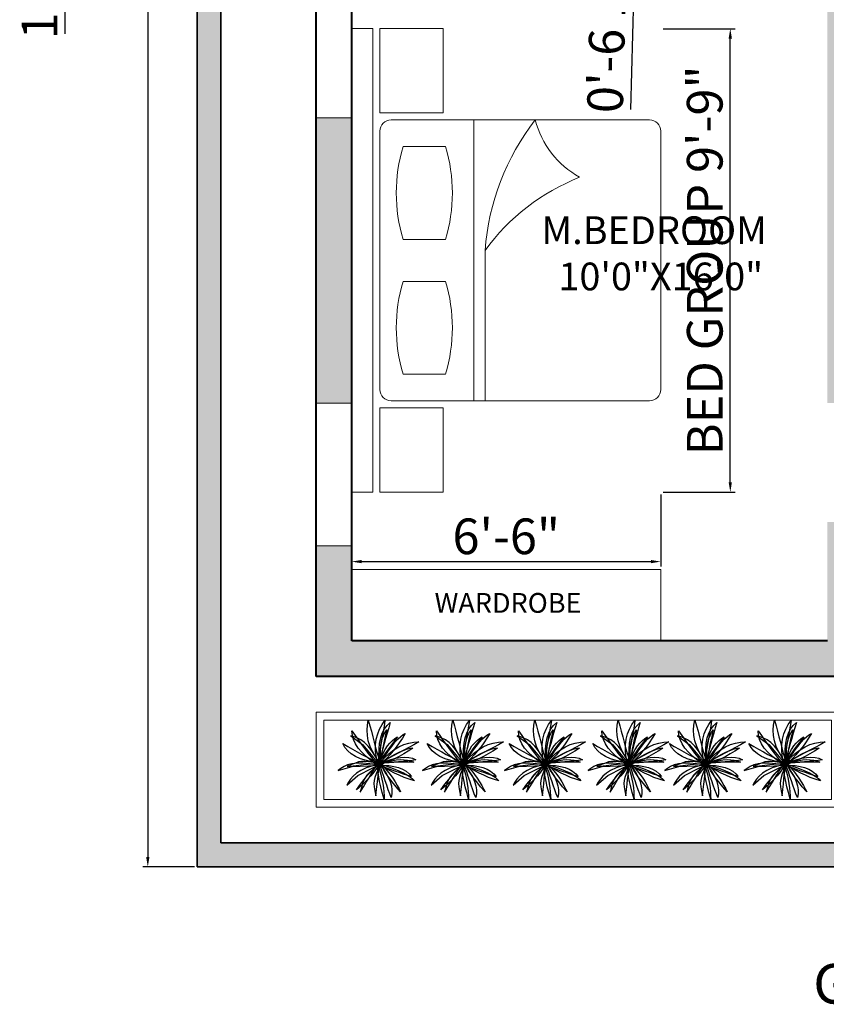
# Model space of a CAD drawing. Units: inches. Extents: x 2337 to 3570, y 1258 to 1938.
# Tile 1 of 30: x 2381 to 2585, y 1258 to 1507. Entities that reach past the tile are written whole.
import ezdxf

# ---------------------------------------------------------------- set-up
doc = ezdxf.new("R2010")
doc.units = ezdxf.units.IN
for name, color, linetype, lineweight in [('A-ANNO-DIMS', 2, 'Continuous', 18), ('A-ANNO-TEXT', 7, 'Continuous', 18), ('A-ANNO-TITL', 7, 'Continuous', 30), ('A-AREA-IDEN', 7, 'Continuous', 18), ('A-FLOR-CASE', 34, 'Continuous', 18), ('A-GLAZ', 4, 'Continuous', 18), ('A-WALL', 7, 'Continuous', 40), ('C-PROP', 7, 'Continuous', 35), ('CAY', 94, 'Continuous', 13), ('furn', 8, 'Continuous', 18), ('L-PLNT-BEDS', 94, 'Continuous', 20)]:
    doc.layers.add(name, color=color, linetype=linetype, lineweight=lineweight)
doc.layers.add('A-WALL-PATT', color=18, linetype='Continuous', lineweight=13, true_color=0x000000)
doc.layers.add('C-PROP-PATT', color=251, linetype='Continuous', lineweight=13, true_color=0x636466)
doc.layers.add('DIENHOA', color=3, linetype='Continuous')
doc.styles.get("Standard").update_dxf_attribs({"font": 'arial.ttf'})
doc.dimstyles.new('ISO-25', dxfattribs={"dimtxt": 9, "dimasz": 2.5, "dimexe": 1.25, "dimexo": 0.625, "dimtad": 1, "dimdec": 1, "dimlunit": 3, "dimtxsty": 'Standard', "dimcen": 2.5, "dimadec": 0, "dimazin": 0, "dimtfac": 1, "dimtdec": 1, "dimtmove": 0, "dimatfit": 3, "dimfxl": 1, "dimarcsym": 0})

# ---------------------------------------------------------------- blocks, each defined once
blk = doc.blocks.new('*D7')
at = {"layer": 'A-ANNO-DIMS', "color": 0, "lineweight": -2, "transparency": 16777216}
for p, q in [((2425.21, 1893.12), (2412.15, 1893.12)), ((2413.4, 1890.62), (2413.4, 1295.62)), ((2425.21, 1293.12), (2412.15, 1293.12))]:
    blk.add_line(p, q, dxfattribs=at)
at = {"layer": 'A-ANNO-DIMS', "color": 0, "transparency": 16777216}
for points in [[(2412.98, 1890.62), (2413.81, 1890.62), (2413.4, 1893.12)], [(2412.98, 1295.62), (2413.81, 1295.62), (2413.4, 1293.12)]]:
    blk.add_solid(points, dxfattribs=at)
at = {"layer": 'Defpoints', "color": 0, "transparency": 16777216}
for p in [(2425.84, 1893.12), (2413.4, 1293.12), (2425.84, 1293.12)]:
    blk.add_point(p, dxfattribs=at)
at = {"layer": 'A-ANNO-DIMS', "color": 0, "transparency": 16777216, "insert": (2408.18, 1593.12), "char_height": 9, "attachment_point": 5, "rotation": 90}
blk.add_mtext("50'", dxfattribs=at)
blk = doc.blocks.new('MAT-P16')
for p, q in [((0, -1.65), (0, 1.65)), ((0, 1.65), (0.15, 1.65)), ((0.15, 1.65), (0.15, -1.65)), ((0.65, 1.65), (0.2, 1.65)), ((0.2, 1.65), (0.2, 1.05)), ((0.65, 1.05), (0.65, 1.65)), ((0.65, 1.05), (0.2, 1.05)), ((2.12, 1), (0.28, 1)), ((0.8695, -1), (0.8695, 1)), ((0.2, 0.92), (0.2, -0.92)), ((2.2, -0.92), (2.2, 0.92)), ((0.6667, 0.8098), (0.3667, 0.8098)), ((0.3667, 0.1498), (0.6667, 0.1498)), ((0.9496, -1), (0.9496, 0.0713)), ((0.3667, -0.1498), (0.6667, -0.1498)), ((0.6667, -0.8098), (0.3667, -0.8098)), ((0.65, -1.05), (0.2, -1.05)), ((0.2, -1.65), (0.2, -1.05)), ((0.28, -1), (2.12, -1)), ((0.65, -1.05), (0.65, -1.65)), ((0.15, -1.65), (0, -1.65)), ((0.65, -1.65), (0.2, -1.65))]:
    blk.add_line(p, q)
for centre, radius, start, end in [((0.28, 0.92), 0.08, 90, 180), ((2.6605, -0.0533), 1.7154, 142.12135, 175.83412), ((1.9461, 1.1681), 0.6614, 194.72006, 240.68633), ((2.12, 0.92), 0.08, 0, 90), ((1.4307, 0.4798), 1.114, 162.7687, 197.2313), ((-0.3973, 0.4798), 1.114, 342.7687, 17.2313), ((2.172, -0.8149), 1.5099, 111.34847, 144.05792), ((1.4307, -0.4798), 1.114, 162.7687, 197.2313), ((-0.3973, -0.4798), 1.114, 342.7687, 17.2313), ((0.28, -0.92), 0.08, 180, 270), ((2.12, -0.92), 0.08, 270, 0)]:
    blk.add_arc(centre, radius, start, end)
blk = doc.blocks.new('Cay03_mb')
at = {"layer": 'DIENHOA'}
for p, q in [((119, 555), (166, 599)), ((166, 599), (142, 519)), ((25, 374), (49, 444)), ((49, 444), (79, 504)), ((79, 504), (119, 555)), ((119, 442), (97, 366)), ((142, 519), (119, 442)), ((-365, 390), (-414, 403)), ((-414, 403), (-240, 278)), ((-315, 371), (-365, 390)), ((-264, 343), (-315, 371)), ((-211, 305), (-264, 343)), ((-158, 252), (-211, 305)), ((2, 206), (10, 295)), ((10, 295), (25, 374)), ((76, 291), (56, 216)), ((97, 366), (76, 291)), ((363, 275), (437, 297)), ((437, 297), (511, 310)), ((511, 310), (586, 314)), ((586, 314), (512, 271)), ((-240, 278), (-88, 95)), ((-104, 184), (-158, 252)), ((-50, 98), (-104, 184)), ((0, 105), (2, 206)), ((56, 216), (37, 142)), ((147, 144), (219, 200)), ((290, 155), (217, 117)), ((219, 200), (291, 243)), ((364, 193), (290, 155)), ((291, 243), (363, 275)), ((438, 231), (364, 193)), ((512, 271), (438, 231)), ((-345, 5), (-400, -17)), ((-299, 20), (-345, 5)), ((-255, 27), (-299, 20)), ((-208, 28), (-255, 27)), ((-153, 22), (-208, 28)), ((-83, 10), (-153, 22)), ((-88, 95), (5, -8)), ((5, -8), (-83, 10)), ((5, -8), (-50, 98)), ((5, -8), (0, 105)), ((5, -8), (76, 75)), ((20, 68), (5, -8)), ((75, 36), (5, -8)), ((5, -8), (100, 18)), ((46, 1), (5, -8)), ((37, 142), (20, 68)), ((97, 7), (46, 1)), ((145, 77), (75, 36)), ((76, 75), (147, 144)), ((155, 12), (97, 7)), ((100, 18), (182, 37)), ((217, 117), (145, 77)), ((220, 15), (155, 12)), ((182, 37), (253, 49)), ((289, 17), (220, 15)), ((253, 49), (315, 54)), ((362, 19), (289, 17)), ((315, 54), (369, 53)), ((436, 19), (362, 19)), ((369, 53), (419, 47)), ((419, 47), (465, 35)), ((510, 19), (436, 19)), ((465, 35), (510, 19)), ((-400, -17), (-468, -48)), ((-468, -48), (-376, -38)), ((-376, -38), (-295, -28)), ((-295, -28), (-226, -19)), ((-226, -19), (-166, -11)), ((-166, -11), (-114, -6)), ((-166, -174), (-120, -122)), ((-120, -122), (-80, -80)), ((-75, -127), (-118, -181)), ((-114, -6), (-69, -3)), ((-80, -80), (-45, -46)), ((-33, -69), (-75, -127)), ((-69, -3), (-30, -3)), ((-45, -46), (-17, -22)), ((5, -8), (-33, -69)), ((-30, -3), (5, -8)), ((-17, -22), (5, -8)), ((5, -8), (57, -73)), ((26, -64), (5, -8)), ((5, -8), (113, -40)), ((53, -42), (5, -8)), ((47, -126), (26, -64)), ((69, -191), (47, -126)), ((107, -76), (53, -42)), ((57, -73), (100, -139)), ((100, -139), (136, -204)), ((166, -110), (107, -76)), ((113, -40), (207, -74)), ((229, -143), (166, -110)), ((207, -74), (290, -108)), ((296, -175), (229, -143)), ((290, -108), (359, -141)), ((359, -141), (417, -174)), ((-271, -307), (-216, -236)), ((-206, -276), (-250, -318)), ((-216, -236), (-166, -174)), ((-162, -231), (-206, -276)), ((-118, -181), (-162, -231)), ((91, -257), (69, -191)), ((113, -322), (91, -257)), ((136, -204), (163, -268)), ((163, -268), (181, -330)), ((367, -205), (296, -175)), ((442, -233), (367, -205)), ((417, -174), (463, -204)), ((519, -258), (442, -233)), ((463, -204), (496, -232)), ((496, -232), (519, -258)), ((-330, -387), (-271, -307)), ((-291, -355), (-330, -387)), ((-250, -318), (-291, -355)), ((135, -386), (113, -322)), ((158, -445), (135, -386)), ((181, -330), (190, -390)), ((190, -390), (190, -446)), ((180, -499), (158, -445)), ((190, -446), (180, -499))]:
    blk.add_line(p, q, dxfattribs=at)
for points in [[(24, -5), (-41, 82), (-92, 167), (-130, 249), (-156, 330), (-170, 408), (-175, 484), (-170, 559), (-157, 633)], [(-157, 633), (-132, 551), (-111, 470), (-90, 389), (-70, 309), (-49, 229), (-27, 150), (-3, 72), (24, -5)], [(-16, -27), (-38, 80), (-49, 178), (-49, 269), (-39, 353), (-19, 430), (9, 501), (45, 567), (88, 629)], [(88, 629), (75, 544), (61, 461), (46, 379), (31, 298), (16, 217), (3, 136), (-8, 55), (-16, -27)], [(-396, 474), (-348, 406), (-301, 339), (-254, 275), (-208, 212), (-162, 151), (-115, 91), (-66, 32), (-16, -27)], [(-16, -27), (-108, 39), (-187, 102), (-252, 163), (-305, 224), (-345, 285), (-374, 347), (-390, 409), (-396, 474)], [(24, -5), (20, 93), (20, 177), (25, 249), (34, 310), (47, 363), (65, 409), (87, 452), (113, 492)], [(113, 492), (96, 420), (79, 347), (64, 276), (50, 208), (38, 145), (30, 87), (25, 36), (24, -5)], [(384, 437), (342, 368), (298, 302), (253, 239), (206, 181), (159, 127), (113, 78), (68, 34), (24, -5)], [(24, -5), (80, 92), (134, 176), (186, 248), (234, 309), (279, 357), (319, 395), (355, 421), (384, 437)], [(-530, 290), (-458, 248), (-388, 208), (-319, 169), (-251, 131), (-183, 95), (-115, 60), (-46, 26), (24, -5)], [(24, -5), (-87, 15), (-185, 40), (-270, 68), (-344, 101), (-406, 140), (-457, 184), (-499, 233), (-530, 290)], [(273, 387), (228, 329), (182, 270), (138, 212), (97, 156), (60, 103), (28, 55), (2, 11), (-16, -27)], [(-16, -27), (21, 64), (57, 140), (91, 203), (125, 255), (160, 297), (195, 332), (233, 362), (273, 387)], [(497, 224), (429, 178), (362, 137), (294, 99), (227, 66), (162, 37), (100, 11), (40, -10), (-16, -27)], [(-16, -27), (75, 38), (160, 92), (237, 136), (307, 170), (368, 195), (420, 213), (463, 222), (497, 224)], [(-16, -27), (-134, -5), (-235, 5), (-322, 5), (-396, -5), (-459, -22), (-512, -46), (-558, -74), (-598, -105)], [(24, -5), (99, 30), (173, 57), (245, 77), (313, 88), (378, 92), (438, 87), (493, 74), (541, 52)], [(541, 52), (484, 43), (421, 35), (354, 28), (285, 21), (216, 14), (148, 8), (83, 2), (24, -5)], [(-598, -105), (-393, -44), (-155, -37), (-16, -27)], [(-472, -320), (-310, -179), (-98, -73), (24, -5)], [(24, -5), (-92, -35), (-188, -68), (-267, -105), (-330, -145), (-380, -187), (-418, -231), (-448, -275), (-472, -320)], [(-276, -424), (-227, -345), (-186, -276), (-150, -216), (-119, -164), (-91, -120), (-66, -82), (-41, -52), (-16, -27)], [(-16, -27), (-85, -86), (-137, -133), (-176, -173), (-204, -210), (-226, -249), (-243, -295), (-258, -352), (-276, -424)], [(24, -5), (-14, -88), (-41, -153), (-60, -205), (-70, -251), (-73, -295), (-69, -344), (-60, -402), (-45, -475)], [(-45, -475), (-34, -383), (-25, -303), (-18, -233), (-12, -173), (-6, -121), (2, -77), (11, -39), (24, -5)], [(76, -524), (49, -428), (27, -342), (9, -264), (-4, -196), (-12, -138), (-17, -90), (-18, -53), (-16, -27)], [(478, -192), (422, -176), (361, -157), (298, -135), (232, -113), (167, -89), (102, -67), (41, -45), (-16, -27)], [(-16, -27), (67, -27), (146, -33), (219, -45), (286, -63), (346, -87), (398, -117), (443, -152), (478, -192)], [(-16, -27), (8, -95), (29, -163), (44, -231), (56, -296), (65, -359), (71, -419), (74, -474), (76, -524)], [(316, -418), (251, -343), (195, -273), (147, -210), (106, -154), (74, -105), (50, -63), (33, -30), (24, -5)], [(24, -5), (75, -57), (122, -111), (164, -165), (203, -219), (237, -273), (267, -324), (294, -373), (316, -418)]]:
    blk.add_lwpolyline(points, dxfattribs=at)
blk = doc.blocks.new('PLANTER-132X24IN')
for points in [[(0, 24), (132, 24), (132, 0), (0, 0)], [(2, 22), (130, 22), (130, 2), (2, 2)]]:
    blk.add_lwpolyline(points, close=True)
blk = doc.blocks.new('*D57')
at = {"layer": 'A-ANNO-DIMS', "color": 0, "lineweight": -2, "transparency": 16777216}
for p, q in [((2534.07, 1539.19), (2537.81, 1539.09)), ((2536.49, 1536.63), (2536.46, 1535.34)), ((2533.91, 1532.9), (2537.65, 1532.81)), ((2536.4, 1532.84), (2535.16, 1484.21))]:
    blk.add_line(p, q, dxfattribs=at)
at = {"layer": 'A-ANNO-DIMS', "color": 0, "transparency": 16777216}
for points in [[(2536.08, 1536.64), (2536.91, 1536.62), (2536.56, 1539.13)], [(2536.04, 1535.35), (2536.88, 1535.33), (2536.4, 1532.84)]]:
    blk.add_solid(points, dxfattribs=at)
at = {"layer": 'Defpoints', "color": 0, "transparency": 16777216}
for p in [(2533.45, 1539.2), (2533.29, 1532.92), (2536.4, 1532.84)]:
    blk.add_point(p, dxfattribs=at)
at = {"layer": 'A-ANNO-DIMS', "color": 0, "transparency": 16777216, "insert": (2530.47, 1507.41), "char_height": 9, "attachment_point": 5, "rotation": 88.5431}
blk.add_mtext('0\'-6 1/2"', dxfattribs=at)
blk = doc.blocks.new('*D84')
at = {"layer": 'A-ANNO-DIMS', "color": 0, "lineweight": -2, "transparency": 16777216}
for p, q in [((2543.41, 1504.58), (2561.58, 1504.58)), ((2560.33, 1390.15), (2560.33, 1502.08)), ((2543.41, 1387.65), (2561.58, 1387.65))]:
    blk.add_line(p, q, dxfattribs=at)
at = {"layer": 'A-ANNO-DIMS', "color": 0, "transparency": 16777216}
for points in [[(2559.91, 1502.08), (2560.74, 1502.08), (2560.33, 1504.58)], [(2559.91, 1390.15), (2560.74, 1390.15), (2560.33, 1387.65)]]:
    blk.add_solid(points, dxfattribs=at)
at = {"layer": 'Defpoints', "color": 0, "transparency": 16777216}
for p in [(2542.79, 1504.58), (2560.33, 1504.58), (2542.79, 1387.65)]:
    blk.add_point(p, dxfattribs=at)
at = {"layer": 'A-ANNO-DIMS', "color": 0, "transparency": 16777216, "insert": (2555.05, 1446.12), "char_height": 9, "attachment_point": 5, "rotation": 90}
blk.add_mtext('BED GROUP 9\'-9"', dxfattribs=at)
blk = doc.blocks.new('*D85')
at = {"layer": 'A-ANNO-DIMS', "color": 0, "lineweight": -2, "transparency": 16777216}
for p, q in [((2464.84, 1387.03), (2464.84, 1368.86)), ((2542.79, 1387.03), (2542.79, 1368.86)), ((2467.34, 1370.11), (2540.29, 1370.11))]:
    blk.add_line(p, q, dxfattribs=at)
at = {"layer": 'A-ANNO-DIMS', "color": 0, "transparency": 16777216}
for points in [[(2467.34, 1370.53), (2467.34, 1369.7), (2464.84, 1370.11)], [(2540.29, 1370.53), (2540.29, 1369.7), (2542.79, 1370.11)]]:
    blk.add_solid(points, dxfattribs=at)
at = {"layer": 'Defpoints', "color": 0, "transparency": 16777216}
for p in [(2464.84, 1387.65), (2542.79, 1387.65), (2542.79, 1370.11)]:
    blk.add_point(p, dxfattribs=at)
at = {"layer": 'A-ANNO-DIMS', "color": 0, "transparency": 16777216, "insert": (2503.81, 1375.33), "char_height": 9, "attachment_point": 5}
blk.add_mtext('6\'-6"', dxfattribs=at)
blk = doc.blocks.new('*D108')
at = {"layer": 'A-ANNO-DIMS', "color": 0, "lineweight": -2, "transparency": 16777216}
for p, q in [((2464.21, 1542.12), (2391.19, 1542.12)), ((2392.44, 1539.62), (2392.44, 1532.62)), ((2464.21, 1530.12), (2391.19, 1530.12)), ((2392.44, 1530.12), (2392.44, 1503.29))]:
    blk.add_line(p, q, dxfattribs=at)
at = {"layer": 'A-ANNO-DIMS', "color": 0, "transparency": 16777216}
for points in [[(2392.02, 1539.62), (2392.85, 1539.62), (2392.44, 1542.12)], [(2392.02, 1532.62), (2392.85, 1532.62), (2392.44, 1530.12)]]:
    blk.add_solid(points, dxfattribs=at)
at = {"layer": 'Defpoints', "color": 0, "transparency": 16777216}
for p in [(2464.84, 1542.12), (2392.44, 1530.12), (2464.84, 1530.12)]:
    blk.add_point(p, dxfattribs=at)
at = {"layer": 'A-ANNO-DIMS', "color": 0, "transparency": 16777216, "insert": (2387.22, 1515.45), "char_height": 9, "attachment_point": 5, "rotation": 90}
blk.add_mtext('1\'-0"', dxfattribs=at)

msp = doc.modelspace()

# ---------------------------------------------------------------- hatches: boundary and pattern name
at = {"layer": 'A-WALL-PATT'}
h = msp.add_hatch(color=256, dxfattribs=at)
h.dxf.hatch_style = 1
h.paths.add_polyline_path([(2671.84, 1857.12), (2455.84, 1857.12), (2455.84, 1824.12), (2464.84, 1824.12), (2464.84, 1848.12), (2671.84, 1848.12)])
h.paths.add_polyline_path([(2566.84, 1764.12), (2464.84, 1764.12), (2464.84, 1788.12), (2455.84, 1788.12), (2455.84, 1743.12), (2464.84, 1743.12), (2464.84, 1755.12), (2566.84, 1755.12)])
h.paths.add_polyline_path([(2683.84, 1761.12), (2683.84, 1764.12), (2602.84, 1764.12), (2602.84, 1755.12), (2608.84, 1755.12), (2608.84, 1701.12), (2662.84, 1701.12), (2662.84, 1605.12), (2671.84, 1605.12), (2671.84, 1713.12), (2662.84, 1713.12), (2662.84, 1707.12), (2614.84, 1707.12), (2614.84, 1755.12), (2662.84, 1755.12), (2662.84, 1749.12), (2671.84, 1749.12), (2671.84, 1755.12), (2683.84, 1755.12)])
h.paths.add_polyline_path([(2464.84, 1707.12), (2455.84, 1707.12), (2455.84, 1617.12), (2464.84, 1617.12), (2464.84, 1635.12), (2506.84, 1635.12), (2506.84, 1641.12), (2464.84, 1641.12)])
h.paths.add_polyline_path([(2542.84, 1551.12), (2464.84, 1551.12), (2464.84, 1569.12), (2455.84, 1569.12), (2455.84, 1518.12), (2464.84, 1518.12), (2464.84, 1542.12), (2542.84, 1542.12)])
h.paths.add_polyline_path([(2464.84, 1482.12), (2455.84, 1482.12), (2455.84, 1410.12), (2464.84, 1410.12)])
h.paths.add_polyline_path([(2626.84, 1350.12), (2590.84, 1350.12), (2590.84, 1380.12), (2584.84, 1380.12), (2584.84, 1350.12), (2464.84, 1350.12), (2464.84, 1374.12), (2455.84, 1374.12), (2455.84, 1341.12), (2626.84, 1341.12)])
h.paths.add_polyline_path([(2662.84, 1416.12), (2686.84, 1416.12), (2686.84, 1422.12), (2590.84, 1422.12), (2590.84, 1542.12), (2680.84, 1542.12), (2680.84, 1551.12), (2671.84, 1551.12), (2671.84, 1557.12), (2662.84, 1557.12), (2662.84, 1551.12), (2578.84, 1551.12), (2578.84, 1542.12), (2584.84, 1542.12), (2584.84, 1410.12), (2590.84, 1410.12), (2590.84, 1416.12), (2656.84, 1416.12), (2656.84, 1350.12), (2650.84, 1350.12), (2650.84, 1341.12), (2731.84, 1341.12), (2731.84, 1362.12), (2722.84, 1362.12), (2722.84, 1350.12), (2662.84, 1350.12)])
h.paths.add_polyline_path([(2731.84, 1434.12), (2722.84, 1434.12), (2722.84, 1422.12), (2716.84, 1422.12), (2716.84, 1416.12), (2722.84, 1416.12), (2722.84, 1386.12), (2731.84, 1386.12)], flags=17)
h.paths.add_polyline_path([(2731.84, 1542.12), (2752.84, 1542.12), (2752.84, 1551.12), (2716.84, 1551.12), (2716.84, 1545.12), (2716.84, 1542.12), (2722.84, 1542.12), (2722.84, 1482.12), (2731.84, 1482.12)])
h.paths.add_polyline_path([(2809.84, 1551.12), (2788.84, 1551.12), (2788.84, 1542.12), (2809.84, 1542.12), (2809.84, 1548.12)])
h.paths.add_polyline_path([(2872.84, 1647.12), (2863.84, 1647.12), (2863.84, 1551.12), (2857.84, 1551.12), (2857.84, 1548.12), (2857.84, 1542.12), (2872.84, 1542.12)])
h.paths.add_polyline_path([(2872.84, 1764.12), (2827.84, 1764.12), (2827.84, 1755.12), (2863.84, 1755.12), (2863.84, 1719.12), (2872.84, 1719.12)])
h.paths.add_polyline_path([(2755.84, 1764.12), (2719.84, 1764.12), (2719.84, 1755.12), (2755.84, 1755.12)])
at = {"layer": 'C-PROP-PATT'}
h = msp.add_hatch(color=256, dxfattribs=at)
h.dxf.hatch_style = 1
h.paths.add_polyline_path([(2905.84, 1893.12), (2425.84, 1893.12), (2425.84, 1293.12), (2731.84, 1293.12), (2731.84, 1299.12), (2431.84, 1299.12), (2431.84, 1887.12), (2899.84, 1887.12), (2899.84, 1875.12), (2905.84, 1875.12)])
h.paths.add_polyline_path([(2845.84, 1299.12), (2827.84, 1299.12), (2827.84, 1293.12), (2845.84, 1293.12)], flags=17)
h.paths.add_polyline_path([(2905.84, 1779.12), (2899.84, 1779.12), (2899.84, 1299.12), (2893.84, 1299.12), (2893.84, 1293.12), (2905.84, 1293.12)], flags=17)

# ---------------------------------------------------------------- linework, layer by layer
at = {"layer": 'A-FLOR-CASE'}
for q in [(2464.84, 1368.12), (2542.84, 1350.12)]:
    msp.add_line((2542.84, 1368.12), q, dxfattribs=at)
at = {"layer": 'A-GLAZ'}
for p, q in [((2464.84, 1482.12), (2455.84, 1482.12)), ((2464.84, 1410.12), (2455.84, 1410.12)), ((2464.84, 1374.12), (2455.84, 1374.12))]:
    msp.add_line(p, q, dxfattribs=at)
at = {"layer": 'A-WALL'}
for p, q in [((2455.84, 1341.12), (2455.84, 1857.12)), ((2464.84, 1350.12), (2464.84, 1542.12)), ((2584.84, 1350.12), (2464.84, 1350.12)), ((2731.84, 1341.12), (2455.84, 1341.12))]:
    msp.add_line(p, q, dxfattribs=at)
at = {"layer": 'C-PROP'}
for p, q in [((2425.84, 1293.12), (2425.84, 1893.12)), ((2431.84, 1299.12), (2431.84, 1887.12)), ((2731.84, 1299.12), (2431.84, 1299.12)), ((2731.84, 1293.12), (2425.84, 1293.12))]:
    msp.add_line(p, q, dxfattribs=at)

# ---------------------------------------------------------------- block references
at = {"layer": 'CAY', "xscale": 0.0172255344823027, "yscale": 0.0172255344823027, "zscale": 0.0172255344823027}
for p in [(2471.71, 1319.21), (2493.02, 1319.21), (2513.71, 1319.21), (2534.75, 1319.21), (2554.1, 1319.21), (2574.16, 1319.21)]:
    msp.add_blockref('Cay03_mb', p, dxfattribs=at)
at = {"layer": 'furn', "xscale": 35.43309000000001, "yscale": 35.43309000000001, "zscale": 35.43309000000001}
msp.add_blockref('MAT-P16', (2464.84, 1446.12), dxfattribs=at)
at = {"layer": 'L-PLNT-BEDS'}
msp.add_blockref('PLANTER-132X24IN', (2455.84, 1308.12), dxfattribs=at)

# ---------------------------------------------------------------- texts
at = {"layer": 'A-ANNO-TEXT', "insert": (2485.74, 1362.19), "char_height": 5, "attachment_point": 1}
msp.add_mtext_dynamic_manual_height_columns('WARDROBE', width=66.911, gutter_width=12.5, heights=[0], dxfattribs=at)
at = {"layer": 'A-ANNO-TITL', "insert": (2581.25, 1268.59), "char_height": 10, "attachment_point": 1}
msp.add_mtext_dynamic_manual_height_columns('GROUND FLOOR PLAN', width=180.1947, gutter_width=12.5, heights=[0], dxfattribs=at)
at = {"layer": 'A-AREA-IDEN', "insert": (2512.69, 1457.23), "char_height": 7, "attachment_point": 1}
msp.add_mtext_dynamic_manual_height_columns('M.BEDROOM\\P  10\'0"X16\'0"', width=66.911, gutter_width=12.5, heights=[0], dxfattribs=at)

# ---------------------------------------------------------------- dimensions: what is measured, and where the dimension line sits
at = {"layer": 'A-ANNO-DIMS'}
for base, p1, p2, angle, override, picture, middle in [((2413.4, 1293.12), (2425.84, 1893.12), (2425.84, 1293.12), 90, {"dimclrd": 0, "dimclre": 0, "dimclrt": 0}, '*D7', (2408.18, 1593.12)), ((2392.44, 1530.12), (2464.84, 1542.12), (2464.84, 1530.12), 90, {"dimdec": 1, "dimlfac": 1, "dimrnd": 0, "dimzin": 1, "dimdsep": 46, "dimlunit": 4, "dimfrac": 2}, '*D108', (2387.22, 1515.45)), ((2536.4, 1532.84), (2533.45, 1539.2), (2533.29, 1532.92), 268.5431, {"dimdec": 1, "dimlfac": 1, "dimrnd": 0, "dimzin": 1, "dimdsep": 46, "dimlunit": 4, "dimfrac": 2}, '*D57', (2530.47, 1507.41))]:
    dim = msp.add_linear_dim(base=base, p1=p1, p2=p2, angle=angle, dimstyle='ISO-25', override=override, dxfattribs=at)
    dim.commit()
    dim.dimension.update_dxf_attribs({"geometry": picture, "text_midpoint": middle})
dim = msp.add_linear_dim(base=(2560.33, 1504.58), p1=(2542.79, 1387.65), p2=(2542.79, 1504.58), angle=90, text='BED GROUP <>', dimstyle='ISO-25', override={"dimdec": 1, "dimlfac": 1, "dimrnd": 0, "dimzin": 1, "dimdsep": 46, "dimlunit": 4, "dimfrac": 2}, dxfattribs=at)
dim.commit()
dim.dimension.update_dxf_attribs({"geometry": '*D84', "text_midpoint": (2555.05, 1446.12)})
dim = msp.add_linear_dim(base=(2542.7886, 1370.112), p1=(2464.8358, 1387.6514), p2=(2542.7886, 1387.6514), dimstyle='ISO-25', override={"dimdec": 1, "dimlfac": 1, "dimrnd": 0, "dimzin": 1, "dimdsep": 46, "dimlunit": 4, "dimfrac": 2}, dxfattribs=at)
dim.commit()
dim.dimension.update_dxf_attribs({"geometry": '*D85', "text_midpoint": (2503.8122, 1375.3322)})

doc.saveas('drawing.dxf')
